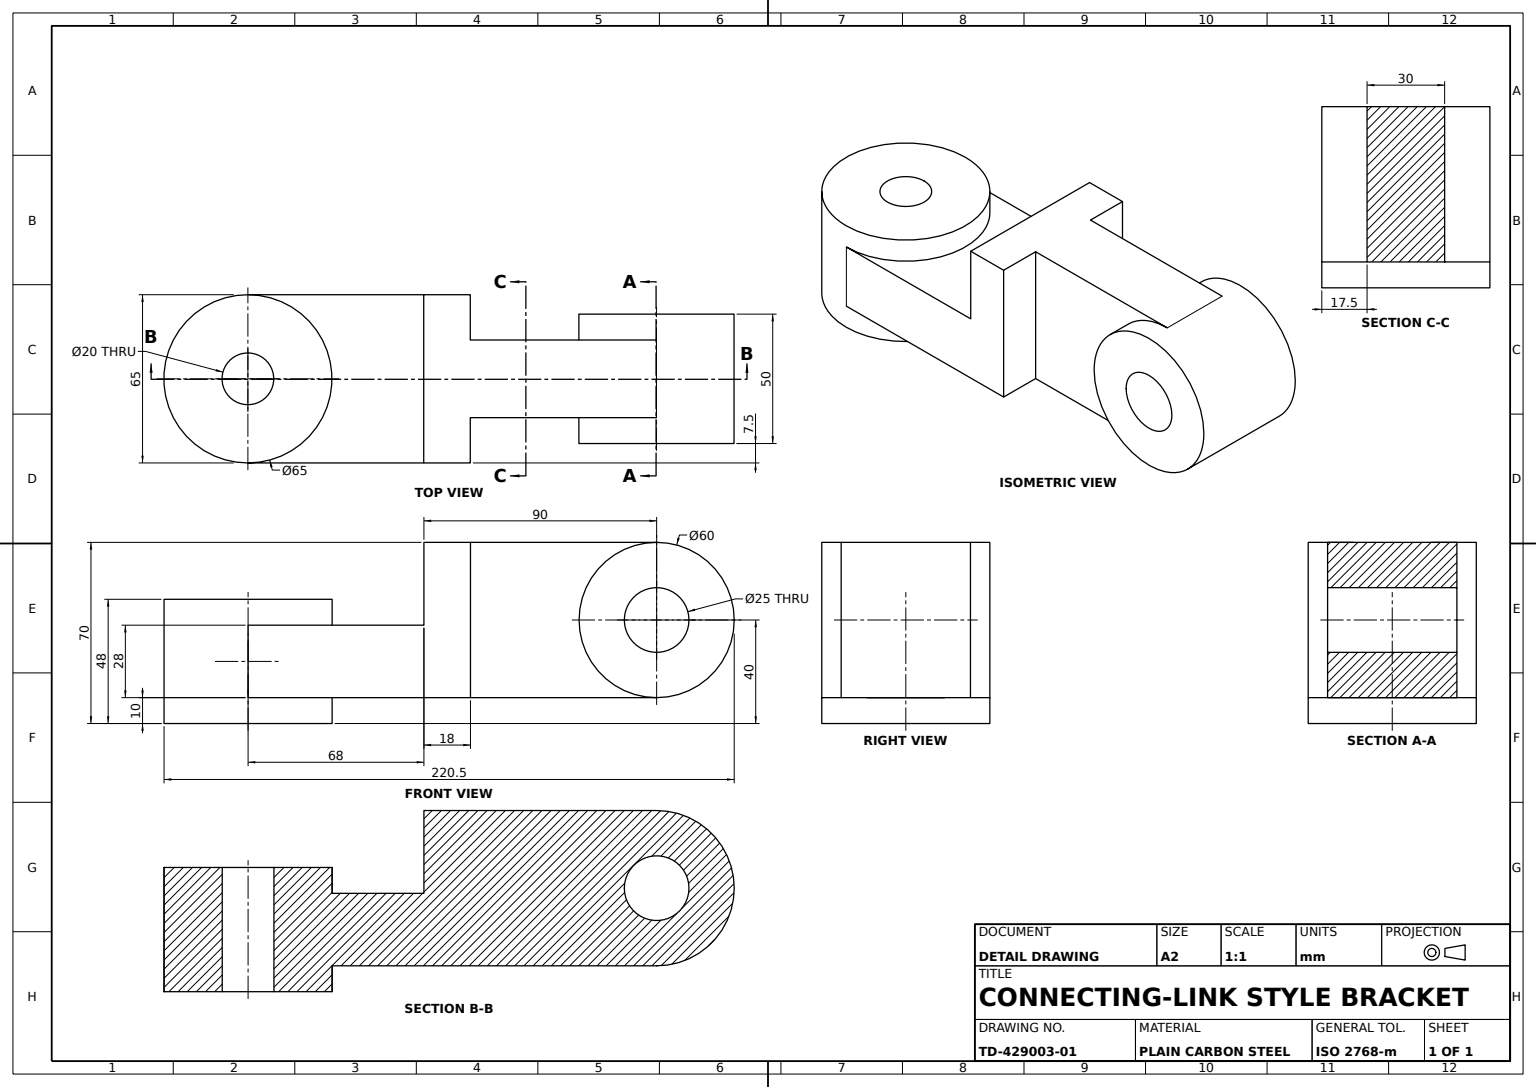
SolidWorks part; units mm, degrees
material "Plain Carbon Steel"
ref_plane "Front Plane" through (0, 0, 0) normal (0, 0, 1) x (1, 0, 0)
ref_plane "Top Plane" through (0, 0, 0) normal (0, 1, 0) x (1, 0, 0)
ref_plane "Right Plane" through (0, 0, 0) normal (1, 0, 0) x (0, 0, -1)
sketch "Main Body Sketch" plane through (0, 0, 0) normal (0, 0, 1) x (1, 0, 0)
  line L0 (0, 0) -> (50, 0)
  line L1 (0, 0) -> (50, 0)
  line L2 (50, 0) -> (50, 32)
  line L3 (50, 32) -> (68, 32)
  line L4 (68, 32) -> (68, -28)
  line L5 (68, -28) -> (0, -28)
  line L6 (0, -28) -> (0, 0)
  dimension "D1" = 50
  dimension "D2" = 68
  dimension "D3" = 28
  dimension "D4" = 60
extrude "Main Body" add sketch "Main Body Sketch" along normal blind 65 contours L6 L5 L4 L3 L2 L0
sketch "Center Pad Sketch" plane through (0, 0, 0) normal (-1, 0, 0) x (0, 0, 1)
  line L0 (0, 0) -> (65, 0)
  line L1 (65, 0) -> (65, -28)
  line L2 (65, -28) -> (0, -28)
  line L3 (0, -28) -> (0, 0)
extrude "Center Pad" add sketch "Center Pad Sketch" along normal blind 18
sketch "Vertical Boss Sketch" plane through (0, 0, 0) normal (0, 1, 0) x (1, 0, 0)
  line L0 (-18, -65) -> (-18, 0) construction
  circle A0 centre (-18, -32.5) radius 32.5
  dimension "D1" = 65
  dimension "D2" = 65
extrude "Vertical Boss" add sketch "Vertical Boss Sketch" against normal blind 48
sketch "Vertical Boss Collar Sketch" plane through (0, 0, 0) normal (0, 1, 0) x (1, 0, 0)
  circle A0 centre (-18, -32.5) radius 32.5
  dimension "D1" = 65
  dimension "D2" = 65
extrude "Vertical Boss Collar" add sketch "Vertical Boss Collar Sketch" along normal blind 10
sketch "Vertical Boss Relief Sketch" plane through (0, -48, 0) normal (0, -1, 0) x (1, 0, 0)
  circle A0 centre (-18, 32.5) radius 32.5
  dimension "D1" = 65
  dimension "D2" = 65
extrude "Vertical Boss Relief Cut" cut sketch "Vertical Boss Relief Sketch" against normal blind 10
sketch "Vertical Bore Sketch" plane through (0, 10, 0) normal (0, 1, 0) x (1, 0, 0)
  circle A0 centre (-18, -32.5) radius 10
  dimension "D1" = 20
  dimension "D2" = 20
extrude "Vertical Bore Ø20" cut sketch "Vertical Bore Sketch" against normal blind 48
sketch "Arm Sketch" plane through (0, 32, 0) normal (0, 1, 0) x (1, 0, 0)
  line L1 (68, -65) -> (68, 0) construction
  line L2 (140, -32.5) -> (140, -17.5)
  line L3 (140, -17.5) -> (68, -17.5)
  line L5 (68, -47.5) -> (140, -47.5)
  line L6 (140, -47.5) -> (140, -32.5)
  line L7 (68, -17.5) -> (68, -47.5)
  line L8 (50, -65) -> (50, 0) construction
  line L9 (50, 0) -> (68, 0) construction
  dimension "D1" = 90
  dimension "D2" = 17.5
  dimension "D3" = 32.5
extrude "Arm" add sketch "Arm Sketch" against normal blind 60
sketch "Horizontal Boss Sketch" plane through (0, 0, 47.5) normal (0, 0, 1) x (1, 0, 0)
  line L0 (140, -28) -> (140, 32) construction
  circle A0 centre (140, 2) radius 30
  dimension "D1" = 60
  dimension "D2" = 60
extrude "Horizontal Boss" add sketch "Horizontal Boss Sketch" against normal blind 40
sketch "Horizontal Boss Collar Sketch" plane through (0, 0, 47.5) normal (0, 0, 1) x (1, 0, 0)
  circle A0 centre (140, 2) radius 30
  dimension "D1" = 60
  dimension "D2" = 60
extrude "Horizontal Boss Collar" add sketch "Horizontal Boss Collar Sketch" along normal blind 10
sketch "Horizontal Bore Sketch" plane through (0, 0, 57.5) normal (0, 0, 1) x (1, 0, 0)
  circle A0 centre (140, 2) radius 12.5
  dimension "D1" = 25
  dimension "D2" = 25
extrude "Horizontal Bore Ø25" cut sketch "Horizontal Bore Sketch" against normal blind 50
